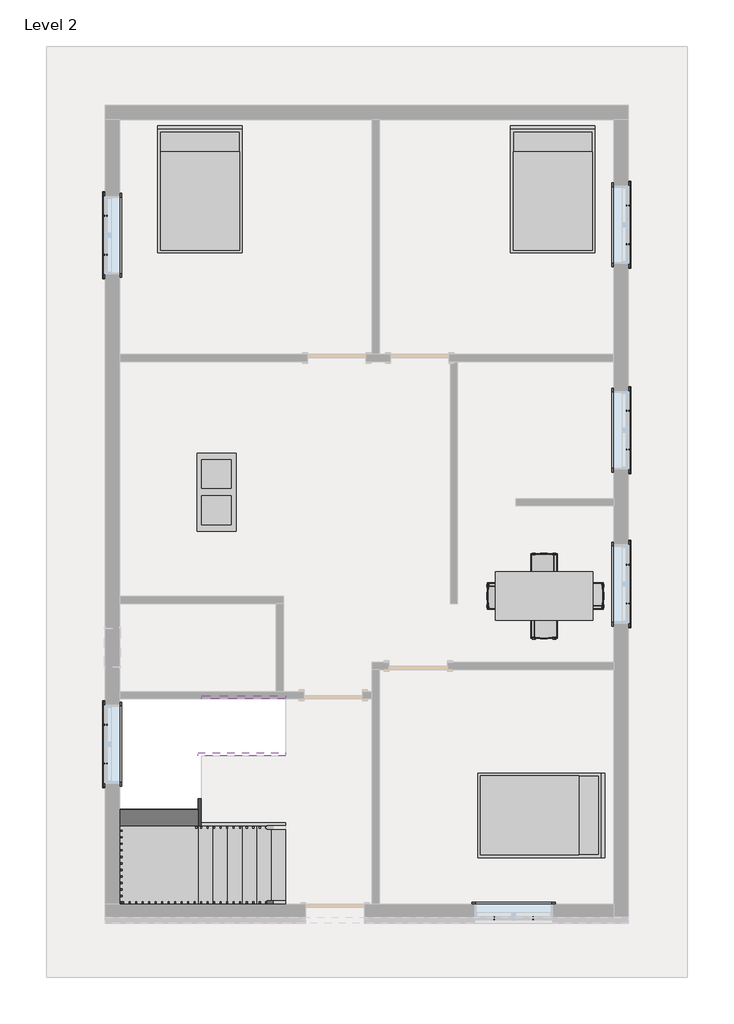
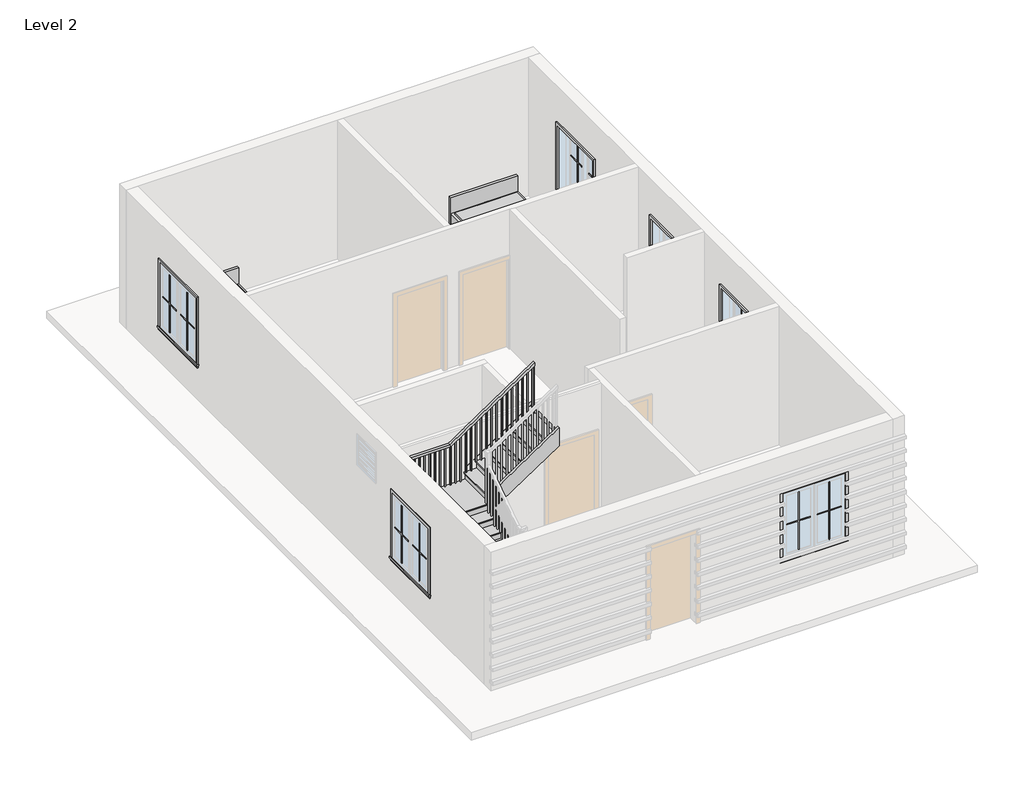
# One storey, part 3 of 3: 25 proxies, 5 members, 4 furniture elements, 1 railing, 1 stair flight.
"""IFC4 building model written with IfcOpenShell, lengths in millimetres."""

from ifc_helpers import new_model, si_unit, frame, origin, place, context, project, spatial, polyline, outline, extrude, faceted_brep, transform, mapped, element, save
from components import muntin_pattern_2x2_muntin_pattern_2x2_ba8901dc, muntin_pattern_2x2_muntin_pattern_2x2_877df4e9, trim_window_exterior_flat_with_sill_fda35bc9, trim_window_interior_flat_picture_frame_a80dbcd9, coffee_table_with_brass_mullions_11320_coffee_table_with_5962bef7, bed_17739_bed_17739_15c61121, dining_table_w_chairs_11374_0cdfc61b, stair_flight_8a4abe09

model = new_model("IFC4")

# Units and contexts
model_context = context("Model", 3, world=origin())
ifc_project = project(units=[si_unit("LENGTHUNIT", "METRE", prefix="MILLI")], contexts=[model_context])

# Site, building, storey
site = spatial("IfcSite", under=ifc_project)
building = spatial("IfcBuilding", under=site)
storey = spatial("IfcBuildingStorey", under=building, Name="Level 2", Elevation=3048.0)

# Proxies
placement = place(None, origin())
muntin_pattern_2x2_muntin_pattern_2x2_shape = muntin_pattern_2x2_muntin_pattern_2x2_ba8901dc(model_context)
element("IfcBuildingElementProxy", 1, Name="Muntin Pattern_2x2 : Muntin Pattern_2x2", ObjectType="Muntin Pattern_2x2 : Muntin Pattern_2x2", at=placement, inside=storey, context=model_context, shape_type="MappedRepresentation", body=[
    mapped(muntin_pattern_2x2_muntin_pattern_2x2_shape, transform((-5325.0867403, -4189.9051559, 4032.25), x_axis=(0.0, 1.0, 0.0), y_axis=(-1.0, 0.0, 0.0), z_axis=(0.0, 0.0, 1.0))),
])
element("IfcBuildingElementProxy", 2, Name="Muntin Pattern_2x2 : Muntin Pattern_2x2", ObjectType="Muntin Pattern_2x2 : Muntin Pattern_2x2", at=placement, inside=storey, context=model_context, shape_type="MappedRepresentation", body=[
    mapped(muntin_pattern_2x2_muntin_pattern_2x2_shape, transform((-5325.0867403, 3744.4198441, 4032.25), x_axis=(0.0, 1.0, 0.0), y_axis=(-1.0, 0.0, 0.0), z_axis=(0.0, 0.0, 1.0))),
])
element("IfcBuildingElementProxy", 3, Name="Muntin Pattern_2x2 : Muntin Pattern_2x2", ObjectType="Muntin Pattern_2x2 : Muntin Pattern_2x2", at=placement, inside=storey, context=model_context, shape_type="MappedRepresentation", body=[
    mapped(muntin_pattern_2x2_muntin_pattern_2x2_shape, transform((2821.9632597, 4512.7698441, 4032.25), x_axis=(0.0, -1.0, 0.0), y_axis=(1.0, 0.0, 0.0), z_axis=(0.0, 0.0, 1.0))),
])
element("IfcBuildingElementProxy", 4, Name="Muntin Pattern_2x2 : Muntin Pattern_2x2", ObjectType="Muntin Pattern_2x2 : Muntin Pattern_2x2", at=placement, inside=storey, context=model_context, shape_type="MappedRepresentation", body=[
    mapped(muntin_pattern_2x2_muntin_pattern_2x2_shape, transform((2821.9632597, 1312.3698441, 4032.25), x_axis=(0.0, -1.0, 0.0), y_axis=(1.0, 0.0, 0.0), z_axis=(0.0, 0.0, 1.0))),
])
element("IfcBuildingElementProxy", 5, Name="Muntin Pattern_2x2 : Muntin Pattern_2x2", ObjectType="Muntin Pattern_2x2 : Muntin Pattern_2x2", at=placement, inside=storey, context=model_context, shape_type="MappedRepresentation", body=[
    mapped(muntin_pattern_2x2_muntin_pattern_2x2_shape, transform((2821.9632597, -1087.9301559, 4032.25), x_axis=(0.0, -1.0, 0.0), y_axis=(1.0, 0.0, 0.0), z_axis=(0.0, 0.0, 1.0))),
])
element("IfcBuildingElementProxy", 6, Name="Muntin Pattern_2x2 : Muntin Pattern_2x2", ObjectType="Muntin Pattern_2x2 : Muntin Pattern_2x2", at=placement, inside=storey, context=model_context, shape_type="MappedRepresentation", body=[
    mapped(muntin_pattern_2x2_muntin_pattern_2x2_shape, transform((1344.0007597, -6601.3176559, 4032.25), x_axis=(-1.0, 0.0, 0.0), y_axis=(0.0, -1.0, 0.0), z_axis=(0.0, 0.0, 1.0))),
])
muntin_pattern_2x2_muntin_pattern_2x2_2_shape = muntin_pattern_2x2_muntin_pattern_2x2_877df4e9(model_context)
element("IfcBuildingElementProxy", 7, Name="Muntin Pattern_2x2 : Muntin Pattern_2x2", ObjectType="Muntin Pattern_2x2 : Muntin Pattern_2x2", at=placement, inside=storey, context=model_context, shape_type="MappedRepresentation", body=[
    mapped(muntin_pattern_2x2_muntin_pattern_2x2_2_shape, transform((-5325.0867403, -3583.4801559, 4032.25), x_axis=(0.0, -1.0, 0.0), y_axis=(1.0, 0.0, 0.0), z_axis=(0.0, 0.0, 1.0))),
])
element("IfcBuildingElementProxy", 8, Name="Muntin Pattern_2x2 : Muntin Pattern_2x2", ObjectType="Muntin Pattern_2x2 : Muntin Pattern_2x2", at=placement, inside=storey, context=model_context, shape_type="MappedRepresentation", body=[
    mapped(muntin_pattern_2x2_muntin_pattern_2x2_2_shape, transform((-5325.0867403, 4350.8448441, 4032.25), x_axis=(0.0, -1.0, 0.0), y_axis=(1.0, 0.0, 0.0), z_axis=(0.0, 0.0, 1.0))),
])
element("IfcBuildingElementProxy", 9, Name="Muntin Pattern_2x2 : Muntin Pattern_2x2", ObjectType="Muntin Pattern_2x2 : Muntin Pattern_2x2", at=placement, inside=storey, context=model_context, shape_type="MappedRepresentation", body=[
    mapped(muntin_pattern_2x2_muntin_pattern_2x2_2_shape, transform((2821.9632597, 3906.3448441, 4032.25), x_axis=(0.0, 1.0, 0.0), y_axis=(-1.0, 0.0, 0.0), z_axis=(0.0, 0.0, 1.0))),
])
element("IfcBuildingElementProxy", 10, Name="Muntin Pattern_2x2 : Muntin Pattern_2x2", ObjectType="Muntin Pattern_2x2 : Muntin Pattern_2x2", at=placement, inside=storey, context=model_context, shape_type="MappedRepresentation", body=[
    mapped(muntin_pattern_2x2_muntin_pattern_2x2_2_shape, transform((2821.9632597, 705.9448441, 4032.25), x_axis=(0.0, 1.0, 0.0), y_axis=(-1.0, 0.0, 0.0), z_axis=(0.0, 0.0, 1.0))),
])
element("IfcBuildingElementProxy", 11, Name="Muntin Pattern_2x2 : Muntin Pattern_2x2", ObjectType="Muntin Pattern_2x2 : Muntin Pattern_2x2", at=placement, inside=storey, context=model_context, shape_type="MappedRepresentation", body=[
    mapped(muntin_pattern_2x2_muntin_pattern_2x2_2_shape, transform((2821.9632597, -1694.3551559, 4032.25), x_axis=(0.0, 1.0, 0.0), y_axis=(-1.0, 0.0, 0.0), z_axis=(0.0, 0.0, 1.0))),
])
element("IfcBuildingElementProxy", 12, Name="Muntin Pattern_2x2 : Muntin Pattern_2x2", ObjectType="Muntin Pattern_2x2 : Muntin Pattern_2x2", at=placement, inside=storey, context=model_context, shape_type="MappedRepresentation", body=[
    mapped(muntin_pattern_2x2_muntin_pattern_2x2_2_shape, transform((737.5757597, -6601.3176559, 4032.25), x_axis=(1.0, 0.0, 0.0), y_axis=(0.0, 1.0, 0.0), z_axis=(0.0, 0.0, 1.0))),
])
trim_window_exterior_flat_with_sill_shape = trim_window_exterior_flat_with_sill_fda35bc9(model_context)
element("IfcBuildingElementProxy", 13, Name="Trim-Window-Exterior-Flat : with Sill", ObjectType="Trim-Window-Exterior-Flat : with Sill", at=placement, inside=storey, context=model_context, shape_type="MappedRepresentation", body=[
    mapped(trim_window_exterior_flat_with_sill_shape, transform((-5334.6117403, -3886.6926559, 5308.6), x_axis=(0.0, -1.0, 0.0), y_axis=(0.0, 0.0, 1.0), z_axis=(-1.0, 0.0, 0.0))),
])
element("IfcBuildingElementProxy", 14, Name="Trim-Window-Exterior-Flat : with Sill", ObjectType="Trim-Window-Exterior-Flat : with Sill", at=placement, inside=storey, context=model_context, shape_type="MappedRepresentation", body=[
    mapped(trim_window_exterior_flat_with_sill_shape, transform((-5334.6117403, 4047.6323441, 5308.6), x_axis=(0.0, -1.0, 0.0), y_axis=(0.0, 0.0, 1.0), z_axis=(-1.0, 0.0, 0.0))),
])
element("IfcBuildingElementProxy", 15, Name="Trim-Window-Exterior-Flat : with Sill", ObjectType="Trim-Window-Exterior-Flat : with Sill", at=placement, inside=storey, context=model_context, shape_type="MappedRepresentation", body=[
    mapped(trim_window_exterior_flat_with_sill_shape, transform((2831.4882597, 4209.5573441, 5308.6), x_axis=(0.0, 1.0, 0.0), y_axis=(0.0, 0.0, 1.0), z_axis=(1.0, 0.0, 0.0))),
])
element("IfcBuildingElementProxy", 16, Name="Trim-Window-Exterior-Flat : with Sill", ObjectType="Trim-Window-Exterior-Flat : with Sill", at=placement, inside=storey, context=model_context, shape_type="MappedRepresentation", body=[
    mapped(trim_window_exterior_flat_with_sill_shape, transform((2831.4882597, 1009.1573441, 5308.6), x_axis=(0.0, 1.0, 0.0), y_axis=(0.0, 0.0, 1.0), z_axis=(1.0, 0.0, 0.0))),
])
element("IfcBuildingElementProxy", 17, Name="Trim-Window-Exterior-Flat : with Sill", ObjectType="Trim-Window-Exterior-Flat : with Sill", at=placement, inside=storey, context=model_context, shape_type="MappedRepresentation", body=[
    mapped(trim_window_exterior_flat_with_sill_shape, transform((2831.4882597, -1391.1426559, 5308.6), x_axis=(0.0, 1.0, 0.0), y_axis=(0.0, 0.0, 1.0), z_axis=(1.0, 0.0, 0.0))),
])
element("IfcBuildingElementProxy", 18, Name="Trim-Window-Exterior-Flat : with Sill", ObjectType="Trim-Window-Exterior-Flat : with Sill", at=placement, inside=storey, context=model_context, shape_type="MappedRepresentation", body=[
    mapped(trim_window_exterior_flat_with_sill_shape, transform((1040.7882597, -6610.8426559, 5308.6), x_axis=(1.0, 0.0, 0.0), y_axis=(0.0, 0.0, 1.0), z_axis=(0.0, -1.0, 0.0))),
])
trim_window_interior_flat_picture_frame_shape = trim_window_interior_flat_picture_frame_a80dbcd9(model_context)
element("IfcBuildingElementProxy", 19, Name="Trim-Window-Interior-Flat : Picture Frame", ObjectType="Trim-Window-Interior-Flat : Picture Frame", at=placement, inside=storey, context=model_context, shape_type="MappedRepresentation", body=[
    mapped(trim_window_interior_flat_picture_frame_shape, transform((-5106.0117403, -3886.6926559, 5308.6), x_axis=(0.0, 1.0, 0.0), y_axis=(0.0, 0.0, 1.0), z_axis=(1.0, 0.0, 0.0))),
])
element("IfcBuildingElementProxy", 20, Name="Trim-Window-Interior-Flat : Picture Frame", ObjectType="Trim-Window-Interior-Flat : Picture Frame", at=placement, inside=storey, context=model_context, shape_type="MappedRepresentation", body=[
    mapped(trim_window_interior_flat_picture_frame_shape, transform((-5106.0117403, 4047.6323441, 5308.6), x_axis=(0.0, 1.0, 0.0), y_axis=(0.0, 0.0, 1.0), z_axis=(1.0, 0.0, 0.0))),
])
element("IfcBuildingElementProxy", 21, Name="Trim-Window-Interior-Flat : Picture Frame", ObjectType="Trim-Window-Interior-Flat : Picture Frame", at=placement, inside=storey, context=model_context, shape_type="MappedRepresentation", body=[
    mapped(trim_window_interior_flat_picture_frame_shape, transform((2602.8882597, 4209.5573441, 5308.6), x_axis=(0.0, -1.0, 0.0), y_axis=(0.0, 0.0, 1.0), z_axis=(-1.0, 0.0, 0.0))),
])
element("IfcBuildingElementProxy", 22, Name="Trim-Window-Interior-Flat : Picture Frame", ObjectType="Trim-Window-Interior-Flat : Picture Frame", at=placement, inside=storey, context=model_context, shape_type="MappedRepresentation", body=[
    mapped(trim_window_interior_flat_picture_frame_shape, transform((2602.8882597, 1009.1573441, 5308.6), x_axis=(0.0, -1.0, 0.0), y_axis=(0.0, 0.0, 1.0), z_axis=(-1.0, 0.0, 0.0))),
])
element("IfcBuildingElementProxy", 23, Name="Trim-Window-Interior-Flat : Picture Frame", ObjectType="Trim-Window-Interior-Flat : Picture Frame", at=placement, inside=storey, context=model_context, shape_type="MappedRepresentation", body=[
    mapped(trim_window_interior_flat_picture_frame_shape, transform((2602.8882597, -1391.1426559, 5308.6), x_axis=(0.0, -1.0, 0.0), y_axis=(0.0, 0.0, 1.0), z_axis=(-1.0, 0.0, 0.0))),
])
element("IfcBuildingElementProxy", 24, Name="Trim-Window-Interior-Flat : Picture Frame", ObjectType="Trim-Window-Interior-Flat : Picture Frame", at=placement, inside=storey, context=model_context, shape_type="MappedRepresentation", body=[
    mapped(trim_window_interior_flat_picture_frame_shape, transform((1040.7882597, -6382.2426559, 5308.6), x_axis=(-1.0, 0.0, 0.0), y_axis=(0.0, 0.0, 1.0), z_axis=(0.0, 1.0, 0.0))),
])
coffee_table_with_brass_mullions_11320_coffee_table_with_shape = coffee_table_with_brass_mullions_11320_coffee_table_with_5962bef7(model_context)
element("IfcBuildingElementProxy", 25, Name="coffee_table_with_brass_mullions_11320 : coffee_table_with_brass_mullions_11320", ObjectType="coffee_table_with_brass_mullions_11320 : coffee_table_with_brass_mullions_11320", at=placement, inside=storey, context=model_context, shape_type="MappedRepresentation", body=[
    mapped(coffee_table_with_brass_mullions_11320_coffee_table_with_shape, transform((-3162.9117403, 678.9573441, 3048.0), x_axis=(0.0, 1.0, 0.0), y_axis=(-1.0, 0.0, 0.0), z_axis=(0.0, 0.0, 1.0))),
])

# Furniture
bed_17739_bed_17739_shape = bed_17739_bed_17739_15c61121(model_context)
element("IfcFurniture", 26, ObjectType="Bed_17739 : Bed_17739", at=placement, inside=storey, context=model_context, shape_type="MappedRepresentation", body=[
    mapped(bed_17739_bed_17739_shape, transform((-3855.0617403, 4742.9573441, 3048.0), x_axis=(1.0, 0.0, 0.0), y_axis=(0.0, 1.0, 0.0), z_axis=(0.0, 0.0, 1.0))),
])
element("IfcFurniture", 27, ObjectType="Bed_17739 : Bed_17739", at=placement, inside=storey, context=model_context, shape_type="MappedRepresentation", body=[
    mapped(bed_17739_bed_17739_shape, transform((1650.3882597, 4742.9573441, 3048.0), x_axis=(1.0, 0.0, 0.0), y_axis=(0.0, 1.0, 0.0), z_axis=(0.0, 0.0, 1.0))),
])
element("IfcFurniture", 28, ObjectType="Bed_17739 : Bed_17739", at=placement, inside=storey, context=model_context, shape_type="MappedRepresentation", body=[
    mapped(bed_17739_bed_17739_shape, transform((1447.1882597, -4997.9426559, 3048.0), x_axis=(0.0, -1.0, 0.0), y_axis=(1.0, 0.0, 0.0), z_axis=(0.0, 0.0, 1.0))),
])
dining_table_w_chairs_11374_shape = dining_table_w_chairs_11374_0cdfc61b(model_context)
element("IfcFurniture", 29, ObjectType="Dining_Table_w_Chairs_11374", at=placement, inside=storey, context=model_context, shape_type="MappedRepresentation", body=[
    mapped(dining_table_w_chairs_11374_shape, transform((1497.0410232, -1671.6886654, 3048.0), x_axis=(1.0, 0.0, 0.0), y_axis=(0.0, 1.0, 0.0), z_axis=(0.0, 0.0, 1.0))),
])

# Members
element("IfcMember", 30, ObjectType="Stringer - 2\" Width", at=placement, inside=storey, context=model_context, shape_type="SweptSolid", body=[
    extrude(outline(polyline([(3048.0, -2515.2117403), (3266.0398409, -2515.2117403), (3520.0398409, -2896.2117403), (3520.0398409, -3445.6977546), (3048.0, -2737.6379933), (3048.0, -2515.2117403)])), frame((0.0, -6433.0426559, 0.0), z_axis=(0.0, 1.0, 0.0), x_axis=(0.0, 0.0, 1.0)), (0.0, 0.0, 1.0), 50.8),
])
element("IfcMember", 31, ObjectType="Stringer - 2\" Width", at=placement, inside=storey, context=model_context, shape_type="SweptSolid", body=[
    extrude(outline(polyline([(5287.3158313, -3277.2117403), (5795.3158313, -2515.2117403), (6161.6398409, -2515.2117403), (5287.3158313, -3826.6977546), (5287.3158313, -3277.2117403)])), frame((0.0, -3181.8426559, 0.0), z_axis=(0.0, 1.0, 0.0), x_axis=(0.0, 0.0, 1.0)), (0.0, 0.0, 1.0), 50.8),
])
element("IfcMember", 32, ObjectType="Stringer - 2\" Width", at=placement, inside=storey, context=model_context, shape_type="SweptSolid", body=[
    extrude(outline(polyline([(3048.0, -2515.2117403), (3266.0398409, -2515.2117403), (4146.5731743, -3836.0117403), (3780.2491647, -3836.0117403), (3048.0, -2737.6379933), (3048.0, -2515.2117403)])), frame((0.0, -5163.0426559, 0.0), z_axis=(0.0, 1.0, 0.0), x_axis=(0.0, 0.0, 1.0)), (0.0, 0.0, 1.0), 50.8),
])
element("IfcMember", 33, ObjectType="Stringer - 2\" Width", at=placement, inside=storey, context=model_context, shape_type="SweptSolid", body=[
    extrude(outline(polyline([(-5163.0426559, 3966.5158313), (-5163.0426559, 4332.8398409), (-4070.8426559, 5060.9731743), (-4070.8426559, 4694.6491647), (-5163.0426559, 3966.5158313)])), frame((-3886.8117403, 0.0, 0.0), z_axis=(1.0, 0.0, 0.0), x_axis=(0.0, 1.0, 0.0)), (0.0, 0.0, 1.0), 50.8),
])
element("IfcMember", 34, ObjectType="Stringer - 2\" Width", at=placement, inside=storey, context=model_context, shape_type="SweptSolid", body=[
    extrude(outline(polyline([(5247.2398409, -3886.8117403), (4880.9158313, -3886.8117403), (5795.3158313, -2515.2117403), (6161.6398409, -2515.2117403), (5247.2398409, -3886.8117403)])), frame((0.0, -4070.8426559, 0.0), z_axis=(0.0, 1.0, 0.0), x_axis=(0.0, 0.0, 1.0)), (0.0, 0.0, 1.0), 50.8),
])

# Railing
element("IfcRailing", 35, ObjectType="Handrail - Rectangular", at=placement, inside=storey, context=model_context, shape_type="SolidModel", body=[
    faceted_brep([(-2515.2117403, -6382.2426559, 4114.8), (-2515.2117403, -6382.2426559, 4053.7459984), (-2515.2117403, -6331.4426559, 4053.7459984), (-2515.2117403, -6331.4426559, 4114.8), (-4001.1117403, -6382.2426559, 5105.4), (-4016.4927427, -6382.2426559, 5054.6), (-4016.4927427, -6331.4426559, 5054.6), (-4001.1117403, -6331.4426559, 5105.4), (-5106.0117403, -6382.2426559, 5105.4), (-5106.0117403, -6382.2426559, 5054.6), (-5055.2117403, -6331.4426559, 5054.6), (-5055.2117403, -6331.4426559, 5105.4), (-5106.0117403, -5277.3426559, 5105.4), (-5106.0117403, -5261.9616535, 5054.6), (-5055.2117403, -5261.9616535, 5054.6), (-5055.2117403, -5277.3426559, 5105.4), (-5106.0117403, -4096.2426559, 5892.8), (-5106.0117403, -4080.8616535, 5842.0), (-5055.2117403, -4080.8616535, 5842.0), (-5055.2117403, -4096.2426559, 5892.8), (-5106.0117403, -3181.8426559, 5892.8), (-5106.0117403, -3181.8426559, 5842.0), (-5055.2117403, -3232.6426559, 5842.0), (-5055.2117403, -3232.6426559, 5892.8), (-4191.6117403, -3181.8426559, 5892.8), (-4176.2307379, -3181.8426559, 5842.0), (-4176.2307379, -3232.6426559, 5842.0), (-4191.6117403, -3232.6426559, 5892.8), (-2515.2117403, -3181.8426559, 7010.4), (-2515.2117403, -3232.6426559, 7010.4), (-2515.2117403, -3232.6426559, 6949.3459984), (-2515.2117403, -3181.8426559, 6949.3459984)], [[[0, 1, 2, 3]], [[1, 0, 4, 5]], [[2, 1, 5, 6]], [[3, 2, 6, 7]], [[0, 3, 7, 4]], [[5, 4, 8, 9]], [[6, 5, 9, 10]], [[7, 6, 10, 11]], [[4, 7, 11, 8]], [[9, 8, 12, 13]], [[10, 9, 13, 14]], [[11, 10, 14, 15]], [[8, 11, 15, 12]], [[13, 12, 16, 17]], [[14, 13, 17, 18]], [[15, 14, 18, 19]], [[12, 15, 19, 16]], [[17, 16, 20, 21]], [[18, 17, 21, 22]], [[19, 18, 22, 23]], [[16, 19, 23, 20]], [[21, 20, 24, 25]], [[22, 21, 25, 26]], [[23, 22, 26, 27]], [[20, 23, 27, 24]], [[28, 29, 30, 31]], [[25, 24, 28, 31]], [[26, 25, 31, 30]], [[27, 26, 30, 29]], [[24, 27, 29, 28]]]),
    extrude(outline(polyline([(6926.0626651, -2550.1367403), (5943.6, -2550.1367403), (5943.6, -2531.0867403), (6938.7626651, -2531.0867403), (6926.0626651, -2550.1367403)])), frame((0.0, -3216.7676559, 0.0), z_axis=(0.0, 1.0, 0.0), x_axis=(0.0, 0.0, 1.0)), (0.0, 0.0, 1.0), 19.05),
    extrude(outline(polyline([(6858.3293317, -2651.7367403), (5943.6, -2651.7367403), (5943.6, -2632.6867403), (6871.0293317, -2632.6867403), (6858.3293317, -2651.7367403)])), frame((0.0, -3216.7676559, 0.0), z_axis=(0.0, 1.0, 0.0), x_axis=(0.0, 0.0, 1.0)), (0.0, 0.0, 1.0), 19.05),
    extrude(outline(polyline([(6790.5959984, -2753.3367403), (5943.6, -2753.3367403), (5943.6, -2734.2867403), (6803.2959984, -2734.2867403), (6790.5959984, -2753.3367403)])), frame((0.0, -3216.7676559, 0.0), z_axis=(0.0, 1.0, 0.0), x_axis=(0.0, 0.0, 1.0)), (0.0, 0.0, 1.0), 19.05),
    extrude(outline(polyline([(6722.8626651, -2854.9367403), (5791.2, -2854.9367403), (5791.2, -2835.8867403), (6735.5626651, -2835.8867403), (6722.8626651, -2854.9367403)])), frame((0.0, -3216.7676559, 0.0), z_axis=(0.0, 1.0, 0.0), x_axis=(0.0, 0.0, 1.0)), (0.0, 0.0, 1.0), 19.05),
    extrude(outline(polyline([(6655.1293317, -2956.5367403), (5791.2, -2956.5367403), (5791.2, -2937.4867403), (6667.8293317, -2937.4867403), (6655.1293317, -2956.5367403)])), frame((0.0, -3216.7676559, 0.0), z_axis=(0.0, 1.0, 0.0), x_axis=(0.0, 0.0, 1.0)), (0.0, 0.0, 1.0), 19.05),
    extrude(outline(polyline([(6587.3959984, -3058.1367403), (5638.8, -3058.1367403), (5638.8, -3039.0867403), (6600.0959984, -3039.0867403), (6587.3959984, -3058.1367403)])), frame((0.0, -3216.7676559, 0.0), z_axis=(0.0, 1.0, 0.0), x_axis=(0.0, 0.0, 1.0)), (0.0, 0.0, 1.0), 19.05),
    extrude(outline(polyline([(6519.6626651, -3159.7367403), (5638.8, -3159.7367403), (5638.8, -3140.6867403), (6532.3626651, -3140.6867403), (6519.6626651, -3159.7367403)])), frame((0.0, -3216.7676559, 0.0), z_axis=(0.0, 1.0, 0.0), x_axis=(0.0, 0.0, 1.0)), (0.0, 0.0, 1.0), 19.05),
    extrude(outline(polyline([(6451.9293317, -3261.3367403), (5486.4, -3261.3367403), (5486.4, -3242.2867403), (6464.6293317, -3242.2867403), (6451.9293317, -3261.3367403)])), frame((0.0, -3216.7676559, 0.0), z_axis=(0.0, 1.0, 0.0), x_axis=(0.0, 0.0, 1.0)), (0.0, 0.0, 1.0), 19.05),
    extrude(outline(polyline([(6384.1959984, -3362.9367403), (5486.4, -3362.9367403), (5486.4, -3343.8867403), (6396.8959984, -3343.8867403), (6384.1959984, -3362.9367403)])), frame((0.0, -3216.7676559, 0.0), z_axis=(0.0, 1.0, 0.0), x_axis=(0.0, 0.0, 1.0)), (0.0, 0.0, 1.0), 19.05),
    extrude(outline(polyline([(6316.4626651, -3464.5367403), (5334.0, -3464.5367403), (5334.0, -3445.4867403), (6329.1626651, -3445.4867403), (6316.4626651, -3464.5367403)])), frame((0.0, -3216.7676559, 0.0), z_axis=(0.0, 1.0, 0.0), x_axis=(0.0, 0.0, 1.0)), (0.0, 0.0, 1.0), 19.05),
    extrude(outline(polyline([(6248.7293317, -3566.1367403), (5334.0, -3566.1367403), (5334.0, -3547.0867403), (6261.4293317, -3547.0867403), (6248.7293317, -3566.1367403)])), frame((0.0, -3216.7676559, 0.0), z_axis=(0.0, 1.0, 0.0), x_axis=(0.0, 0.0, 1.0)), (0.0, 0.0, 1.0), 19.05),
    extrude(outline(polyline([(6180.9959984, -3667.7367403), (5334.0, -3667.7367403), (5334.0, -3648.6867403), (6193.6959984, -3648.6867403), (6180.9959984, -3667.7367403)])), frame((0.0, -3216.7676559, 0.0), z_axis=(0.0, 1.0, 0.0), x_axis=(0.0, 0.0, 1.0)), (0.0, 0.0, 1.0), 19.05),
    extrude(outline(polyline([(6113.2626651, -3769.3367403), (5181.6, -3769.3367403), (5181.6, -3750.2867403), (6125.9626651, -3750.2867403), (6113.2626651, -3769.3367403)])), frame((0.0, -3216.7676559, 0.0), z_axis=(0.0, 1.0, 0.0), x_axis=(0.0, 0.0, 1.0)), (0.0, 0.0, 1.0), 19.05),
    extrude(outline(polyline([(6045.5293317, -3870.9367403), (5181.6, -3870.9367403), (5181.6, -3851.8867403), (6058.2293317, -3851.8867403), (6045.5293317, -3870.9367403)])), frame((0.0, -3216.7676559, 0.0), z_axis=(0.0, 1.0, 0.0), x_axis=(0.0, 0.0, 1.0)), (0.0, 0.0, 1.0), 19.05),
    extrude(outline(polyline([(5977.7959984, -3972.5367403), (5029.2, -3972.5367403), (5029.2, -3953.4867403), (5990.4959984, -3953.4867403), (5977.7959984, -3972.5367403)])), frame((0.0, -3216.7676559, 0.0), z_axis=(0.0, 1.0, 0.0), x_axis=(0.0, 0.0, 1.0)), (0.0, 0.0, 1.0), 19.05),
    extrude(outline(polyline([(5910.0626651, -4074.1367403), (5029.2, -4074.1367403), (5029.2, -4055.0867403), (5922.7626651, -4055.0867403), (5910.0626651, -4074.1367403)])), frame((0.0, -3216.7676559, 0.0), z_axis=(0.0, 1.0, 0.0), x_axis=(0.0, 0.0, 1.0)), (0.0, 0.0, 1.0), 19.05),
    extrude(outline(polyline([(5842.3293317, -4175.7367403), (5029.2, -4175.7367403), (5029.2, -4156.6867403), (5855.0293317, -4156.6867403), (5842.3293317, -4175.7367403)])), frame((0.0, -3216.7676559, 0.0), z_axis=(0.0, 1.0, 0.0), x_axis=(0.0, 0.0, 1.0)), (0.0, 0.0, 1.0), 19.05),
    extrude(outline(polyline([(-4277.3367403, -3197.7176559), (-4258.2867403, -3197.7176559), (-4258.2867403, -3216.7676559), (-4277.3367403, -3216.7676559), (-4277.3367403, -3197.7176559)])), frame((0.0, 0.0, 5029.2), z_axis=(0.0, 0.0, 1.0), x_axis=(1.0, 0.0, 0.0)), (0.0, 0.0, 1.0), 812.8),
    extrude(outline(polyline([(-4378.9367403, -3197.7176559), (-4359.8867403, -3197.7176559), (-4359.8867403, -3216.7676559), (-4378.9367403, -3216.7676559), (-4378.9367403, -3197.7176559)])), frame((0.0, 0.0, 5029.2), z_axis=(0.0, 0.0, 1.0), x_axis=(1.0, 0.0, 0.0)), (0.0, 0.0, 1.0), 812.8),
    extrude(outline(polyline([(-4480.5367403, -3197.7176559), (-4461.4867403, -3197.7176559), (-4461.4867403, -3216.7676559), (-4480.5367403, -3216.7676559), (-4480.5367403, -3197.7176559)])), frame((0.0, 0.0, 5029.2), z_axis=(0.0, 0.0, 1.0), x_axis=(1.0, 0.0, 0.0)), (0.0, 0.0, 1.0), 812.8),
    extrude(outline(polyline([(-4582.1367403, -3197.7176559), (-4563.0867403, -3197.7176559), (-4563.0867403, -3216.7676559), (-4582.1367403, -3216.7676559), (-4582.1367403, -3197.7176559)])), frame((0.0, 0.0, 5029.2), z_axis=(0.0, 0.0, 1.0), x_axis=(1.0, 0.0, 0.0)), (0.0, 0.0, 1.0), 812.8),
    extrude(outline(polyline([(-4683.7367403, -3197.7176559), (-4664.6867403, -3197.7176559), (-4664.6867403, -3216.7676559), (-4683.7367403, -3216.7676559), (-4683.7367403, -3197.7176559)])), frame((0.0, 0.0, 5029.2), z_axis=(0.0, 0.0, 1.0), x_axis=(1.0, 0.0, 0.0)), (0.0, 0.0, 1.0), 812.8),
    extrude(outline(polyline([(-4785.3367403, -3197.7176559), (-4766.2867403, -3197.7176559), (-4766.2867403, -3216.7676559), (-4785.3367403, -3216.7676559), (-4785.3367403, -3197.7176559)])), frame((0.0, 0.0, 5029.2), z_axis=(0.0, 0.0, 1.0), x_axis=(1.0, 0.0, 0.0)), (0.0, 0.0, 1.0), 812.8),
    extrude(outline(polyline([(-4886.9367403, -3197.7176559), (-4867.8867403, -3197.7176559), (-4867.8867403, -3216.7676559), (-4886.9367403, -3216.7676559), (-4886.9367403, -3197.7176559)])), frame((0.0, 0.0, 5029.2), z_axis=(0.0, 0.0, 1.0), x_axis=(1.0, 0.0, 0.0)), (0.0, 0.0, 1.0), 812.8),
    extrude(outline(polyline([(-4988.5367403, -3197.7176559), (-4969.4867403, -3197.7176559), (-4969.4867403, -3216.7676559), (-4988.5367403, -3216.7676559), (-4988.5367403, -3197.7176559)])), frame((0.0, 0.0, 5029.2), z_axis=(0.0, 0.0, 1.0), x_axis=(1.0, 0.0, 0.0)), (0.0, 0.0, 1.0), 812.8),
    extrude(outline(polyline([(-5090.1367403, -3318.3676559), (-5090.1367403, -3299.3176559), (-5071.0867403, -3299.3176559), (-5071.0867403, -3318.3676559), (-5090.1367403, -3318.3676559)])), frame((0.0, 0.0, 5029.2), z_axis=(0.0, 0.0, 1.0), x_axis=(1.0, 0.0, 0.0)), (0.0, 0.0, 1.0), 812.8),
    extrude(outline(polyline([(-5090.1367403, -3419.9676559), (-5090.1367403, -3400.9176559), (-5071.0867403, -3400.9176559), (-5071.0867403, -3419.9676559), (-5090.1367403, -3419.9676559)])), frame((0.0, 0.0, 5029.2), z_axis=(0.0, 0.0, 1.0), x_axis=(1.0, 0.0, 0.0)), (0.0, 0.0, 1.0), 812.8),
    extrude(outline(polyline([(-5090.1367403, -3521.5676559), (-5090.1367403, -3502.5176559), (-5071.0867403, -3502.5176559), (-5071.0867403, -3521.5676559), (-5090.1367403, -3521.5676559)])), frame((0.0, 0.0, 5029.2), z_axis=(0.0, 0.0, 1.0), x_axis=(1.0, 0.0, 0.0)), (0.0, 0.0, 1.0), 812.8),
    extrude(outline(polyline([(-5090.1367403, -3623.1676559), (-5090.1367403, -3604.1176559), (-5071.0867403, -3604.1176559), (-5071.0867403, -3623.1676559), (-5090.1367403, -3623.1676559)])), frame((0.0, 0.0, 5029.2), z_axis=(0.0, 0.0, 1.0), x_axis=(1.0, 0.0, 0.0)), (0.0, 0.0, 1.0), 812.8),
    extrude(outline(polyline([(-5090.1367403, -3724.7676559), (-5090.1367403, -3705.7176559), (-5071.0867403, -3705.7176559), (-5071.0867403, -3724.7676559), (-5090.1367403, -3724.7676559)])), frame((0.0, 0.0, 5029.2), z_axis=(0.0, 0.0, 1.0), x_axis=(1.0, 0.0, 0.0)), (0.0, 0.0, 1.0), 812.8),
    extrude(outline(polyline([(-5090.1367403, -3826.3676559), (-5090.1367403, -3807.3176559), (-5071.0867403, -3807.3176559), (-5071.0867403, -3826.3676559), (-5090.1367403, -3826.3676559)])), frame((0.0, 0.0, 5029.2), z_axis=(0.0, 0.0, 1.0), x_axis=(1.0, 0.0, 0.0)), (0.0, 0.0, 1.0), 812.8),
    extrude(outline(polyline([(-5090.1367403, -3927.9676559), (-5090.1367403, -3908.9176559), (-5071.0867403, -3908.9176559), (-5071.0867403, -3927.9676559), (-5090.1367403, -3927.9676559)])), frame((0.0, 0.0, 5029.2), z_axis=(0.0, 0.0, 1.0), x_axis=(1.0, 0.0, 0.0)), (0.0, 0.0, 1.0), 812.8),
    extrude(outline(polyline([(-5090.1367403, -4029.5676559), (-5090.1367403, -4010.5176559), (-5071.0867403, -4010.5176559), (-5071.0867403, -4029.5676559), (-5090.1367403, -4029.5676559)])), frame((0.0, 0.0, 5029.2), z_axis=(0.0, 0.0, 1.0), x_axis=(1.0, 0.0, 0.0)), (0.0, 0.0, 1.0), 812.8),
    extrude(outline(polyline([(-4112.1176559, 5821.1626651), (-4112.1176559, 4876.8), (-4131.1676559, 4876.8), (-4131.1676559, 5808.4626651), (-4112.1176559, 5821.1626651)])), frame((-5090.1367403, 0.0, 0.0), z_axis=(1.0, 0.0, 0.0), x_axis=(0.0, 1.0, 0.0)), (0.0, 0.0, 1.0), 19.05),
    extrude(outline(polyline([(-4213.7176559, 5753.4293317), (-4213.7176559, 4876.8), (-4232.7676559, 4876.8), (-4232.7676559, 5740.7293317), (-4213.7176559, 5753.4293317)])), frame((-5090.1367403, 0.0, 0.0), z_axis=(1.0, 0.0, 0.0), x_axis=(0.0, 1.0, 0.0)), (0.0, 0.0, 1.0), 19.05),
    extrude(outline(polyline([(-4315.3176559, 5685.6959984), (-4315.3176559, 4724.4), (-4334.3676559, 4724.4), (-4334.3676559, 5672.9959984), (-4315.3176559, 5685.6959984)])), frame((-5090.1367403, 0.0, 0.0), z_axis=(1.0, 0.0, 0.0), x_axis=(0.0, 1.0, 0.0)), (0.0, 0.0, 1.0), 19.05),
    extrude(outline(polyline([(-4416.9176559, 5617.9626651), (-4416.9176559, 4724.4), (-4435.9676559, 4724.4), (-4435.9676559, 5605.2626651), (-4416.9176559, 5617.9626651)])), frame((-5090.1367403, 0.0, 0.0), z_axis=(1.0, 0.0, 0.0), x_axis=(0.0, 1.0, 0.0)), (0.0, 0.0, 1.0), 19.05),
    extrude(outline(polyline([(-4518.5176559, 5550.2293317), (-4518.5176559, 4572.0), (-4537.5676559, 4572.0), (-4537.5676559, 5537.5293317), (-4518.5176559, 5550.2293317)])), frame((-5090.1367403, 0.0, 0.0), z_axis=(1.0, 0.0, 0.0), x_axis=(0.0, 1.0, 0.0)), (0.0, 0.0, 1.0), 19.05),
    extrude(outline(polyline([(-4620.1176559, 5482.4959984), (-4620.1176559, 4572.0), (-4639.1676559, 4572.0), (-4639.1676559, 5469.7959984), (-4620.1176559, 5482.4959984)])), frame((-5090.1367403, 0.0, 0.0), z_axis=(1.0, 0.0, 0.0), x_axis=(0.0, 1.0, 0.0)), (0.0, 0.0, 1.0), 19.05),
    extrude(outline(polyline([(-4721.7176559, 5414.7626651), (-4721.7176559, 4419.6), (-4740.7676559, 4419.6), (-4740.7676559, 5402.0626651), (-4721.7176559, 5414.7626651)])), frame((-5090.1367403, 0.0, 0.0), z_axis=(1.0, 0.0, 0.0), x_axis=(0.0, 1.0, 0.0)), (0.0, 0.0, 1.0), 19.05),
    extrude(outline(polyline([(-4823.3176559, 5347.0293317), (-4823.3176559, 4419.6), (-4842.3676559, 4419.6), (-4842.3676559, 5334.3293317), (-4823.3176559, 5347.0293317)])), frame((-5090.1367403, 0.0, 0.0), z_axis=(1.0, 0.0, 0.0), x_axis=(0.0, 1.0, 0.0)), (0.0, 0.0, 1.0), 19.05),
    extrude(outline(polyline([(-4924.9176559, 5279.2959984), (-4924.9176559, 4419.6), (-4943.9676559, 4419.6), (-4943.9676559, 5266.5959984), (-4924.9176559, 5279.2959984)])), frame((-5090.1367403, 0.0, 0.0), z_axis=(1.0, 0.0, 0.0), x_axis=(0.0, 1.0, 0.0)), (0.0, 0.0, 1.0), 19.05),
    extrude(outline(polyline([(-5026.5176559, 5211.5626651), (-5026.5176559, 4267.2), (-5045.5676559, 4267.2), (-5045.5676559, 5198.8626651), (-5026.5176559, 5211.5626651)])), frame((-5090.1367403, 0.0, 0.0), z_axis=(1.0, 0.0, 0.0), x_axis=(0.0, 1.0, 0.0)), (0.0, 0.0, 1.0), 19.05),
    extrude(outline(polyline([(-5128.1176559, 5143.8293317), (-5128.1176559, 4267.2), (-5147.1676559, 4267.2), (-5147.1676559, 5131.1293317), (-5128.1176559, 5143.8293317)])), frame((-5090.1367403, 0.0, 0.0), z_axis=(1.0, 0.0, 0.0), x_axis=(0.0, 1.0, 0.0)), (0.0, 0.0, 1.0), 19.05),
    extrude(outline(polyline([(-5229.7176559, 5076.0959984), (-5229.7176559, 4114.8), (-5248.7676559, 4114.8), (-5248.7676559, 5063.3959984), (-5229.7176559, 5076.0959984)])), frame((-5090.1367403, 0.0, 0.0), z_axis=(1.0, 0.0, 0.0), x_axis=(0.0, 1.0, 0.0)), (0.0, 0.0, 1.0), 19.05),
    extrude(outline(polyline([(-5090.1367403, -5350.3676559), (-5090.1367403, -5331.3176559), (-5071.0867403, -5331.3176559), (-5071.0867403, -5350.3676559), (-5090.1367403, -5350.3676559)])), frame((0.0, 0.0, 4114.8), z_axis=(0.0, 0.0, 1.0), x_axis=(1.0, 0.0, 0.0)), (0.0, 0.0, 1.0), 939.8),
    extrude(outline(polyline([(-5090.1367403, -5451.9676559), (-5090.1367403, -5432.9176559), (-5071.0867403, -5432.9176559), (-5071.0867403, -5451.9676559), (-5090.1367403, -5451.9676559)])), frame((0.0, 0.0, 4114.8), z_axis=(0.0, 0.0, 1.0), x_axis=(1.0, 0.0, 0.0)), (0.0, 0.0, 1.0), 939.8),
    extrude(outline(polyline([(-5090.1367403, -5553.5676559), (-5090.1367403, -5534.5176559), (-5071.0867403, -5534.5176559), (-5071.0867403, -5553.5676559), (-5090.1367403, -5553.5676559)])), frame((0.0, 0.0, 4114.8), z_axis=(0.0, 0.0, 1.0), x_axis=(1.0, 0.0, 0.0)), (0.0, 0.0, 1.0), 939.8),
    extrude(outline(polyline([(-5090.1367403, -5655.1676559), (-5090.1367403, -5636.1176559), (-5071.0867403, -5636.1176559), (-5071.0867403, -5655.1676559), (-5090.1367403, -5655.1676559)])), frame((0.0, 0.0, 4114.8), z_axis=(0.0, 0.0, 1.0), x_axis=(1.0, 0.0, 0.0)), (0.0, 0.0, 1.0), 939.8),
    extrude(outline(polyline([(-5090.1367403, -5756.7676559), (-5090.1367403, -5737.7176559), (-5071.0867403, -5737.7176559), (-5071.0867403, -5756.7676559), (-5090.1367403, -5756.7676559)])), frame((0.0, 0.0, 4114.8), z_axis=(0.0, 0.0, 1.0), x_axis=(1.0, 0.0, 0.0)), (0.0, 0.0, 1.0), 939.8),
    extrude(outline(polyline([(-5090.1367403, -5858.3676559), (-5090.1367403, -5839.3176559), (-5071.0867403, -5839.3176559), (-5071.0867403, -5858.3676559), (-5090.1367403, -5858.3676559)])), frame((0.0, 0.0, 4114.8), z_axis=(0.0, 0.0, 1.0), x_axis=(1.0, 0.0, 0.0)), (0.0, 0.0, 1.0), 939.8),
    extrude(outline(polyline([(-5090.1367403, -5959.9676559), (-5090.1367403, -5940.9176559), (-5071.0867403, -5940.9176559), (-5071.0867403, -5959.9676559), (-5090.1367403, -5959.9676559)])), frame((0.0, 0.0, 4114.8), z_axis=(0.0, 0.0, 1.0), x_axis=(1.0, 0.0, 0.0)), (0.0, 0.0, 1.0), 939.8),
    extrude(outline(polyline([(-5090.1367403, -6061.5676559), (-5090.1367403, -6042.5176559), (-5071.0867403, -6042.5176559), (-5071.0867403, -6061.5676559), (-5090.1367403, -6061.5676559)])), frame((0.0, 0.0, 4114.8), z_axis=(0.0, 0.0, 1.0), x_axis=(1.0, 0.0, 0.0)), (0.0, 0.0, 1.0), 939.8),
    extrude(outline(polyline([(-5090.1367403, -6163.1676559), (-5090.1367403, -6144.1176559), (-5071.0867403, -6144.1176559), (-5071.0867403, -6163.1676559), (-5090.1367403, -6163.1676559)])), frame((0.0, 0.0, 4114.8), z_axis=(0.0, 0.0, 1.0), x_axis=(1.0, 0.0, 0.0)), (0.0, 0.0, 1.0), 939.8),
    extrude(outline(polyline([(-5090.1367403, -6264.7676559), (-5090.1367403, -6245.7176559), (-5071.0867403, -6245.7176559), (-5071.0867403, -6264.7676559), (-5090.1367403, -6264.7676559)])), frame((0.0, 0.0, 4114.8), z_axis=(0.0, 0.0, 1.0), x_axis=(1.0, 0.0, 0.0)), (0.0, 0.0, 1.0), 939.8),
    extrude(outline(polyline([(-5045.6867403, -6366.3676559), (-5064.7367403, -6366.3676559), (-5064.7367403, -6347.3176559), (-5045.6867403, -6347.3176559), (-5045.6867403, -6366.3676559)])), frame((0.0, 0.0, 4114.8), z_axis=(0.0, 0.0, 1.0), x_axis=(1.0, 0.0, 0.0)), (0.0, 0.0, 1.0), 939.8),
    extrude(outline(polyline([(-4944.0867403, -6366.3676559), (-4963.1367403, -6366.3676559), (-4963.1367403, -6347.3176559), (-4944.0867403, -6347.3176559), (-4944.0867403, -6366.3676559)])), frame((0.0, 0.0, 4114.8), z_axis=(0.0, 0.0, 1.0), x_axis=(1.0, 0.0, 0.0)), (0.0, 0.0, 1.0), 939.8),
    extrude(outline(polyline([(-4842.4867403, -6366.3676559), (-4861.5367403, -6366.3676559), (-4861.5367403, -6347.3176559), (-4842.4867403, -6347.3176559), (-4842.4867403, -6366.3676559)])), frame((0.0, 0.0, 4114.8), z_axis=(0.0, 0.0, 1.0), x_axis=(1.0, 0.0, 0.0)), (0.0, 0.0, 1.0), 939.8),
    extrude(outline(polyline([(-4740.8867403, -6366.3676559), (-4759.9367403, -6366.3676559), (-4759.9367403, -6347.3176559), (-4740.8867403, -6347.3176559), (-4740.8867403, -6366.3676559)])), frame((0.0, 0.0, 4114.8), z_axis=(0.0, 0.0, 1.0), x_axis=(1.0, 0.0, 0.0)), (0.0, 0.0, 1.0), 939.8),
    extrude(outline(polyline([(-4639.2867403, -6366.3676559), (-4658.3367403, -6366.3676559), (-4658.3367403, -6347.3176559), (-4639.2867403, -6347.3176559), (-4639.2867403, -6366.3676559)])), frame((0.0, 0.0, 4114.8), z_axis=(0.0, 0.0, 1.0), x_axis=(1.0, 0.0, 0.0)), (0.0, 0.0, 1.0), 939.8),
    extrude(outline(polyline([(-4537.6867403, -6366.3676559), (-4556.7367403, -6366.3676559), (-4556.7367403, -6347.3176559), (-4537.6867403, -6347.3176559), (-4537.6867403, -6366.3676559)])), frame((0.0, 0.0, 4114.8), z_axis=(0.0, 0.0, 1.0), x_axis=(1.0, 0.0, 0.0)), (0.0, 0.0, 1.0), 939.8),
    extrude(outline(polyline([(-4436.0867403, -6366.3676559), (-4455.1367403, -6366.3676559), (-4455.1367403, -6347.3176559), (-4436.0867403, -6347.3176559), (-4436.0867403, -6366.3676559)])), frame((0.0, 0.0, 4114.8), z_axis=(0.0, 0.0, 1.0), x_axis=(1.0, 0.0, 0.0)), (0.0, 0.0, 1.0), 939.8),
    extrude(outline(polyline([(-4334.4867403, -6366.3676559), (-4353.5367403, -6366.3676559), (-4353.5367403, -6347.3176559), (-4334.4867403, -6347.3176559), (-4334.4867403, -6366.3676559)])), frame((0.0, 0.0, 4114.8), z_axis=(0.0, 0.0, 1.0), x_axis=(1.0, 0.0, 0.0)), (0.0, 0.0, 1.0), 939.8),
    extrude(outline(polyline([(-4232.8867403, -6366.3676559), (-4251.9367403, -6366.3676559), (-4251.9367403, -6347.3176559), (-4232.8867403, -6347.3176559), (-4232.8867403, -6366.3676559)])), frame((0.0, 0.0, 4114.8), z_axis=(0.0, 0.0, 1.0), x_axis=(1.0, 0.0, 0.0)), (0.0, 0.0, 1.0), 939.8),
    extrude(outline(polyline([(-4131.2867403, -6366.3676559), (-4150.3367403, -6366.3676559), (-4150.3367403, -6347.3176559), (-4131.2867403, -6347.3176559), (-4131.2867403, -6366.3676559)])), frame((0.0, 0.0, 4114.8), z_axis=(0.0, 0.0, 1.0), x_axis=(1.0, 0.0, 0.0)), (0.0, 0.0, 1.0), 939.8),
    extrude(outline(polyline([(-4029.6867403, -6366.3676559), (-4048.7367403, -6366.3676559), (-4048.7367403, -6347.3176559), (-4029.6867403, -6347.3176559), (-4029.6867403, -6366.3676559)])), frame((0.0, 0.0, 4114.8), z_axis=(0.0, 0.0, 1.0), x_axis=(1.0, 0.0, 0.0)), (0.0, 0.0, 1.0), 939.8),
    extrude(outline(polyline([(5008.3626651, -3947.1367403), (4114.8, -3947.1367403), (4114.8, -3928.0867403), (4995.6626651, -3928.0867403), (5008.3626651, -3947.1367403)])), frame((0.0, -6366.3676559, 0.0), z_axis=(0.0, 1.0, 0.0), x_axis=(0.0, 0.0, 1.0)), (0.0, 0.0, 1.0), 19.05),
    extrude(outline(polyline([(4940.6293317, -3845.5367403), (3962.4, -3845.5367403), (3962.4, -3826.4867403), (4927.9293317, -3826.4867403), (4940.6293317, -3845.5367403)])), frame((0.0, -6366.3676559, 0.0), z_axis=(0.0, 1.0, 0.0), x_axis=(0.0, 0.0, 1.0)), (0.0, 0.0, 1.0), 19.05),
    extrude(outline(polyline([(4872.8959984, -3743.9367403), (3962.4, -3743.9367403), (3962.4, -3724.8867403), (4860.1959984, -3724.8867403), (4872.8959984, -3743.9367403)])), frame((0.0, -6366.3676559, 0.0), z_axis=(0.0, 1.0, 0.0), x_axis=(0.0, 0.0, 1.0)), (0.0, 0.0, 1.0), 19.05),
    extrude(outline(polyline([(4805.1626651, -3642.3367403), (3810.0, -3642.3367403), (3810.0, -3623.2867403), (4792.4626651, -3623.2867403), (4805.1626651, -3642.3367403)])), frame((0.0, -6366.3676559, 0.0), z_axis=(0.0, 1.0, 0.0), x_axis=(0.0, 0.0, 1.0)), (0.0, 0.0, 1.0), 19.05),
    extrude(outline(polyline([(4737.4293317, -3540.7367403), (3810.0, -3540.7367403), (3810.0, -3521.6867403), (4724.7293317, -3521.6867403), (4737.4293317, -3540.7367403)])), frame((0.0, -6366.3676559, 0.0), z_axis=(0.0, 1.0, 0.0), x_axis=(0.0, 0.0, 1.0)), (0.0, 0.0, 1.0), 19.05),
    extrude(outline(polyline([(4669.6959984, -3439.1367403), (3810.0, -3439.1367403), (3810.0, -3420.0867403), (4656.9959984, -3420.0867403), (4669.6959984, -3439.1367403)])), frame((0.0, -6366.3676559, 0.0), z_axis=(0.0, 1.0, 0.0), x_axis=(0.0, 0.0, 1.0)), (0.0, 0.0, 1.0), 19.05),
    extrude(outline(polyline([(4601.9626651, -3337.5367403), (3657.6, -3337.5367403), (3657.6, -3318.4867403), (4589.2626651, -3318.4867403), (4601.9626651, -3337.5367403)])), frame((0.0, -6366.3676559, 0.0), z_axis=(0.0, 1.0, 0.0), x_axis=(0.0, 0.0, 1.0)), (0.0, 0.0, 1.0), 19.05),
    extrude(outline(polyline([(4534.2293317, -3235.9367403), (3657.6, -3235.9367403), (3657.6, -3216.8867403), (4521.5293317, -3216.8867403), (4534.2293317, -3235.9367403)])), frame((0.0, -6366.3676559, 0.0), z_axis=(0.0, 1.0, 0.0), x_axis=(0.0, 0.0, 1.0)), (0.0, 0.0, 1.0), 19.05),
    extrude(outline(polyline([(4466.4959984, -3134.3367403), (3505.2, -3134.3367403), (3505.2, -3115.2867403), (4453.7959984, -3115.2867403), (4466.4959984, -3134.3367403)])), frame((0.0, -6366.3676559, 0.0), z_axis=(0.0, 1.0, 0.0), x_axis=(0.0, 0.0, 1.0)), (0.0, 0.0, 1.0), 19.05),
    extrude(outline(polyline([(4398.7626651, -3032.7367403), (3505.2, -3032.7367403), (3505.2, -3013.6867403), (4386.0626651, -3013.6867403), (4398.7626651, -3032.7367403)])), frame((0.0, -6366.3676559, 0.0), z_axis=(0.0, 1.0, 0.0), x_axis=(0.0, 0.0, 1.0)), (0.0, 0.0, 1.0), 19.05),
    extrude(outline(polyline([(4331.0293317, -2931.1367403), (3352.8, -2931.1367403), (3352.8, -2912.0867403), (4318.3293317, -2912.0867403), (4331.0293317, -2931.1367403)])), frame((0.0, -6366.3676559, 0.0), z_axis=(0.0, 1.0, 0.0), x_axis=(0.0, 0.0, 1.0)), (0.0, 0.0, 1.0), 19.05),
    extrude(outline(polyline([(4263.2959984, -2829.5367403), (3352.8, -2829.5367403), (3352.8, -2810.4867403), (4250.5959984, -2810.4867403), (4263.2959984, -2829.5367403)])), frame((0.0, -6366.3676559, 0.0), z_axis=(0.0, 1.0, 0.0), x_axis=(0.0, 0.0, 1.0)), (0.0, 0.0, 1.0), 19.05),
    extrude(outline(polyline([(4195.5626651, -2727.9367403), (3200.4, -2727.9367403), (3200.4, -2708.8867403), (4182.8626651, -2708.8867403), (4195.5626651, -2727.9367403)])), frame((0.0, -6366.3676559, 0.0), z_axis=(0.0, 1.0, 0.0), x_axis=(0.0, 0.0, 1.0)), (0.0, 0.0, 1.0), 19.05),
    extrude(outline(polyline([(4127.8293317, -2626.3367403), (3200.4, -2626.3367403), (3200.4, -2607.2867403), (4115.1293317, -2607.2867403), (4127.8293317, -2626.3367403)])), frame((0.0, -6366.3676559, 0.0), z_axis=(0.0, 1.0, 0.0), x_axis=(0.0, 0.0, 1.0)), (0.0, 0.0, 1.0), 19.05),
    extrude(outline(polyline([(-5090.1367403, -3216.7676559), (-5090.1367403, -3197.7176559), (-5071.0867403, -3197.7176559), (-5071.0867403, -3216.7676559), (-5090.1367403, -3216.7676559)])), frame((0.0, 0.0, 5029.2), z_axis=(0.0, 0.0, 1.0), x_axis=(1.0, 0.0, 0.0)), (0.0, 0.0, 1.0), 812.8),
    extrude(outline(polyline([(-5071.0867403, -6366.3676559), (-5090.1367403, -6366.3676559), (-5090.1367403, -6347.3176559), (-5071.0867403, -6347.3176559), (-5071.0867403, -6366.3676559)])), frame((0.0, 0.0, 4114.8), z_axis=(0.0, 0.0, 1.0), x_axis=(1.0, 0.0, 0.0)), (0.0, 0.0, 1.0), 939.8),
    extrude(outline(polyline([(6936.6459984, -2534.2617403), (5943.6, -2534.2617403), (5943.6, -2515.2117403), (6949.3459984, -2515.2117403), (6936.6459984, -2534.2617403)])), frame((0.0, -3216.7676559, 0.0), z_axis=(0.0, 1.0, 0.0), x_axis=(0.0, 0.0, 1.0)), (0.0, 0.0, 1.0), 19.05),
    extrude(outline(polyline([(4066.4459984, -2534.2617403), (3200.4, -2534.2617403), (3200.4, -2515.2117403), (4053.7459984, -2515.2117403), (4066.4459984, -2534.2617403)])), frame((0.0, -6366.3676559, 0.0), z_axis=(0.0, 1.0, 0.0), x_axis=(0.0, 0.0, 1.0)), (0.0, 0.0, 1.0), 19.05),
])

# Stair flight
stair_flight_shape = stair_flight_8a4abe09(model_context)
element("IfcStairFlight", 36, ObjectType="2\" Tread 1\" Nosing 1/4\" Riser", at=placement, inside=storey, context=model_context, shape_type="MappedRepresentation", body=[
    mapped(stair_flight_shape, transform((0.0, 0.0, 0.0), x_axis=(1.0, 0.0, 0.0), y_axis=(0.0, 1.0, 0.0), z_axis=(0.0, 0.0, 1.0))),
])

save(model, "model.ifc")

# Revit data of these elements
# Type "Muntin Pattern_2x2 : Muntin Pattern_2x2"
#   Width [instance default] = 4' - 0"
#   Thickness = 0' - 0 1/2"
#   Height [instance default] = 4' - 0"
#   Distance = 0' - 0 3/4"
#   Interior Material [instance default] = none
#   Exterior Material [instance default] = none
#   Default Elevation = 0
# Type "Trim-Window-Exterior-Flat : with Sill"
#   Trim Width = 0' - 2 1/4"
#   Trim Thickness_Picture Frame = 0' - 1 1/4"
#   Trim Thickness_with Sill = 0' - 0 3/4"
#   Sill Thickness = 0' - 1 1/4"
#   Opening Width [instance default] = 2' - 0"
#   Opening Height [instance default] = 3' - 0"
#   Default Elevation = 4' - 0"
#   Sill = yes
#   Picture Frame = no
#   Trim Material [instance default] = none
# Type "Trim-Window-Interior-Flat : Picture Frame"
#   Trim Thickness_Picture Frame = 0' - 1 1/4"
#   Trim Width = 0' - 2 1/4"
#   Trim Thickness_with Sill = 0' - 0 3/4"
#   Sill Thickness = 0' - 1 1/4"
#   Opening Width [instance default] = 2' - 0"
#   Opening Height [instance default] = 3' - 0"
#   Default Elevation = 4' - 0"
#   Sill = no
#   Picture Frame = yes
#   Trim Material [instance default] = none
# Type "coffee_table_with_brass_mullions_11320 : coffee_table_with_brass_mullions_11320"
#   Default Elevation = 0
# Type "Bed_17739 : Bed_17739"
#   Default Elevation = 0
# Type "Dining_Table_w_Chairs_11374"
#   Default Elevation = 0
#   Assembly Code = ""
# Type "Handrail - Rectangular"
#   Assembly Code = "C2010400"
#   built-in parameter 1008612 = 0.0416667 (stored number, unit not read)
#   built-in parameter 1008611 = 0.0416667 (stored number, unit not read)
#   built-in parameter 1008609 = 0.333333 (stored number, unit not read)
#   built-in parameter 1008604 = 0.166667 (stored number, unit not read)
#   built-in parameter 1008603 = 0.166667 (stored number, unit not read)
#   Railing Height = 3' - 0"
#   built-in parameter 1008630 = 2
#   built-in parameter 1008610 = 2
#   built-in parameter 1008618 = Baluster - Square : 3/4"
# Elements 1, 2, 3, 4, 5, 6, 7, 8, 9, 10, 11, 12 (IfcBuildingElementProxy, "Muntin Pattern_2x2 : Muntin Pattern_2x2")
#   Width = 1' - 6 5/8"
#   Height = 3' - 11 1/2"
#   Interior Material = Wood - Stained
#   Exterior Material = Clad - White
#   Phase Created = New Construction
#   Materials on its faces: "Clad - White", "Wood - Stained"
# Elements 13, 14, 15, 16, 17, 18 (IfcBuildingElementProxy, "Trim-Window-Exterior-Flat : with Sill")
#   Opening Width = 4' - 0"
#   Opening Height = 4' - 5"
#   Trim Material = Clad - White
#   Phase Created = New Construction
#   Materials on its faces: "Clad - White"
# Elements 19, 20, 21, 22, 23, 24 (IfcBuildingElementProxy, "Trim-Window-Interior-Flat : Picture Frame")
#   Opening Width = 4' - 0"
#   Opening Height = 4' - 5"
#   Trim Material = Wood - Stained
#   Phase Created = New Construction
#   Materials on its faces: "Wood - Stained"
# Element 25 (IfcBuildingElementProxy, "coffee_table_with_brass_mullions_11320 : coffee_table_with_brass_mullions_11320")
#   Phase Created = New Construction
#   Materials on its faces: "Default Wall", "TABLE", "Glass", "Default"
# Elements 26, 27, 28 (IfcFurniture, "Bed_17739 : Bed_17739")
#   Phase Created = New Construction
#   Materials on its faces: "legs", "sheets", "bed frame", "Blanket"
# Element 29 (IfcFurniture, "Dining_Table_w_Chairs_11374")
#   Phase Created = New Construction
# Elements 30, 31, 32, 33, 34 (IfcMember, "Stringer - 2\" Width")
#   Phase Created = New Construction
# Element 35 (IfcRailing, "Handrail - Rectangular")
#   Phase Created = New Construction
#   Materials on its faces: "Clad - White"
# Element 36 (IfcStairFlight, "2\" Tread 1\" Nosing 1/4\" Riser")
#   Phase Created = New Construction
#   Materials on its faces: "Wood Planks"
# Materials
#   "Clad - White": class "Wood", colour RGB 242 242 238, transparency 0, Cost = 0
#   "Wood - Stained": class "Wood", colour RGB 224 178 126, transparency 0, Cost = 0
#   "Default Wall": colour RGB 128 128 128, transparency 0, Cost = 0
#   "TABLE": class "Generic", colour RGB 120 120 120, transparency 0, Cost = 0
#   "Glass": class "Glass", colour RGB 0 128 192, transparency 0.75, Description = "Soda Lime Glass", Cost = 0
#   "Default": colour RGB 127 127 127, transparency 0, Cost = 0
#   "legs": colour RGB 90 73 37, transparency 0, Cost = 0
#   "sheets": colour RGB 200 195 176, transparency 0, Cost = 0
#   "bed frame": colour RGB 90 73 37, transparency 0, Cost = 0
#   "Blanket": class "System", colour RGB 59 0 1, transparency 0, Cost = 0
#   "Wood Planks": class "Wood", colour RGB 193 160 115, transparency 0, Description = "Physical material.", Cost = 0
